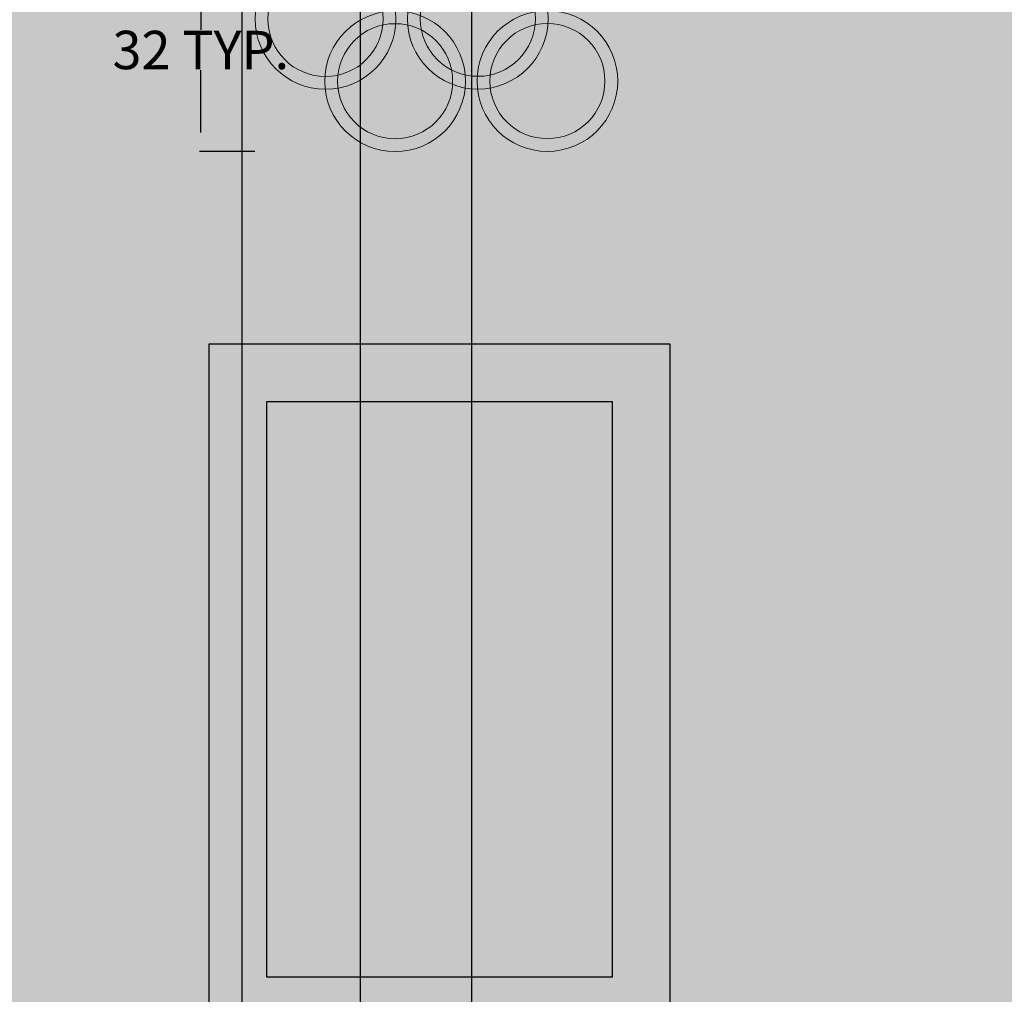
# Model space of a CAD drawing. Units: inches. Extents: x 126 to 726, y 86 to 888.
# Tile 3 of 13: x 270 to 424, y 202 to 354. Entities that reach past the tile are written whole.
import ezdxf

# ---------------------------------------------------------------- set-up
doc = ezdxf.new("R2010")
doc.units = ezdxf.units.IN
doc.header["$MEASUREMENT"] = 0
for name, color, linetype, lineweight in [('A-ANNO-DIMS', 2, 'Continuous', 18), ('A-ELEV-DECO', 7, 'Continuous', 18), ('A-ELEV-PATT', 8, 'Continuous', 13), ('A-GLAZ', 4, 'Continuous', 25)]:
    doc.layers.add(name, color=color, linetype=linetype, lineweight=lineweight)
doc.styles.get("Standard").update_dxf_attribs({"font": 'arial.ttf'})
doc.dimstyles.get("Standard").update_dxf_attribs({"dimtxt": 6, "dimasz": 3, "dimexe": 0.18, "dimexo": 0.0625, "dimgap": 0.09, "dimtad": 0, "dimtih": 1, "dimtoh": 1, "dimdec": 0, "dimzin": 0, "dimdsep": 46, "dimlunit": 3, "dimtxsty": 'Standard', "dimcen": 0.09, "dimadec": 0, "dimazin": 0, "dimtfac": 1, "dimtdec": 0, "dimtofl": 0, "dimtmove": 0, "dimatfit": 3, "dimfxl": 1, "dimtolj": 1, "dimtzin": 0, "dimarcsym": 0})

# ---------------------------------------------------------------- blocks, each defined once
blk = doc.blocks.new('WIN-FRAME')
for points in [[(72, 0), (0, 0), (0, 108), (72, 108)], [(63, 9), (9, 9), (9, 99), (63, 99)]]:
    blk.add_lwpolyline(points, close=True)
blk = doc.blocks.new('MOTIF-RINGS')
for centre, radius in [((11, 20.74), 11), ((34.81, 20.77), 11), ((11, 20.74), 9), ((34.81, 20.77), 9), ((21.88, 11), 11), ((45.69, 11.03), 11), ((45.69, 11.03), 9), ((21.88, 11), 9)]:
    blk.add_circle(centre, radius)
blk = doc.blocks.new('*D9')
at = {"layer": 'A-ANNO-DIMS', "color": 0, "lineweight": -2, "transparency": 16777216}
for p, q in [((306.84, 365.49), (306.84, 374.11)), ((363.53, 365.49), (363.53, 374.11)), ((306.84, 373.93), (303.84, 373.93)), ((360.53, 373.93), (309.84, 373.93))]:
    blk.add_line(p, q, dxfattribs=at)
at = {"layer": 'A-ANNO-DIMS', "color": 0, "transparency": 16777216}
for points in [[(309.84, 374.43), (309.84, 373.43), (306.84, 373.93)], [(360.53, 374.43), (360.53, 373.43), (363.53, 373.93)]]:
    blk.add_solid(points, dxfattribs=at)
at = {"layer": 'Defpoints', "color": 0, "transparency": 16777216}
for p in [(306.84, 373.93), (306.84, 365.42), (363.53, 365.42)]:
    blk.add_point(p, dxfattribs=at)
at = {"layer": 'A-ANNO-DIMS', "color": 0, "transparency": 16777216, "insert": (235.05, 373.93), "char_height": 6, "attachment_point": 5}
blk.add_mtext('\\A1;DECORATIVE RING MOTIF 57 TYP.', dxfattribs=at)
blk = doc.blocks.new('*D10')
at = {"layer": 'A-ANNO-DIMS', "color": 0, "lineweight": -2, "transparency": 16777216}
for p, q in [((306.78, 365.42), (298.16, 365.42)), ((298.34, 362.42), (298.34, 352.7)), ((298.34, 336.66), (298.34, 346.38)), ((306.78, 333.66), (298.16, 333.66))]:
    blk.add_line(p, q, dxfattribs=at)
at = {"layer": 'A-ANNO-DIMS', "color": 0, "transparency": 16777216}
for points in [[(297.84, 362.42), (298.84, 362.42), (298.34, 365.42)], [(297.84, 336.66), (298.84, 336.66), (298.34, 333.66)]]:
    blk.add_solid(points, dxfattribs=at)
at = {"layer": 'Defpoints', "color": 0, "transparency": 16777216}
for p in [(306.84, 365.42), (298.34, 333.66), (306.84, 333.66)]:
    blk.add_point(p, dxfattribs=at)
at = {"layer": 'A-ANNO-DIMS', "color": 0, "transparency": 16777216, "insert": (298.34, 349.54), "char_height": 6, "attachment_point": 5}
blk.add_mtext('\\A1;32 TYP.', dxfattribs=at)
blk = doc.blocks.new('*D13')
at = {"layer": 'A-ANNO-DIMS', "color": 0, "lineweight": -2, "transparency": 16777216}
for p, q in [((665.97, 642.98), (665.97, 90.21)), ((185.97, 126.98), (185.97, 90.21)), ((188.97, 90.39), (419.15, 90.39)), ((662.97, 90.39), (432.8, 90.39))]:
    blk.add_line(p, q, dxfattribs=at)
at = {"layer": 'A-ANNO-DIMS', "color": 0, "transparency": 16777216}
for points in [[(188.97, 90.89), (188.97, 89.89), (185.97, 90.39)], [(662.97, 90.89), (662.97, 89.89), (665.97, 90.39)]]:
    blk.add_solid(points, dxfattribs=at)
at = {"layer": 'Defpoints', "color": 0, "transparency": 16777216}
for p in [(665.97, 643.04), (185.97, 127.04), (665.97, 90.39)]:
    blk.add_point(p, dxfattribs=at)
at = {"layer": 'A-ANNO-DIMS', "color": 0, "transparency": 16777216, "insert": (425.97, 90.39), "char_height": 6, "attachment_point": 5}
blk.add_mtext('\\A1;480', dxfattribs=at)
blk = doc.blocks.new('*D16')
at = {"layer": 'A-ANNO-DIMS', "color": 0, "lineweight": -2, "transparency": 16777216}
for p, q in [((299.6, 425.68), (149.14, 425.68)), ((149.32, 422.68), (149.32, 313.79)), ((149.32, 198.59), (149.32, 307.48)), ((299.6, 195.59), (149.14, 195.59))]:
    blk.add_line(p, q, dxfattribs=at)
at = {"layer": 'A-ANNO-DIMS', "color": 0, "transparency": 16777216}
for points in [[(148.82, 422.68), (149.82, 422.68), (149.32, 425.68)], [(148.82, 198.59), (149.82, 198.59), (149.32, 195.59)]]:
    blk.add_solid(points, dxfattribs=at)
at = {"layer": 'Defpoints', "color": 0, "transparency": 16777216}
for p in [(149.32, 425.68), (299.67, 425.68), (299.67, 195.59)]:
    blk.add_point(p, dxfattribs=at)
at = {"layer": 'A-ANNO-DIMS', "color": 0, "transparency": 16777216, "insert": (149.32, 310.64), "char_height": 6, "attachment_point": 5}
blk.add_mtext('\\A1;230.1', dxfattribs=at)
blk = doc.blocks.new('*D18')
at = {"layer": 'A-ANNO-DIMS', "color": 0, "lineweight": -2, "transparency": 16777216}
for p, q in [((431.28, 395.58), (149.14, 395.58)), ((149.32, 392.58), (149.32, 264.47)), ((149.32, 130.04), (149.32, 258.16)), ((185.91, 127.04), (149.14, 127.04))]:
    blk.add_line(p, q, dxfattribs=at)
at = {"layer": 'A-ANNO-DIMS', "color": 0, "transparency": 16777216}
for points in [[(148.82, 392.58), (149.82, 392.58), (149.32, 395.58)], [(148.82, 130.04), (149.82, 130.04), (149.32, 127.04)]]:
    blk.add_solid(points, dxfattribs=at)
at = {"layer": 'Defpoints', "color": 0, "transparency": 16777216}
for p in [(149.32, 395.58), (431.34, 395.58), (185.97, 127.04)]:
    blk.add_point(p, dxfattribs=at)
at = {"layer": 'A-ANNO-DIMS', "color": 0, "transparency": 16777216, "insert": (149.32, 261.31), "char_height": 6, "attachment_point": 5}
blk.add_mtext('\\A1;268.54', dxfattribs=at)
blk = doc.blocks.new('*D38')
at = {"layer": 'A-ANNO-DIMS', "color": 0, "lineweight": -2, "transparency": 16777216}
for p, q in [((304.8, 168.3), (304.8, 883.87)), ((307.8, 883.69), (320.3, 883.69)), ((323.3, 174.45), (323.3, 883.87)), ((323.3, 883.69), (326.3, 883.69))]:
    blk.add_line(p, q, dxfattribs=at)
at = {"layer": 'A-ANNO-DIMS', "color": 0, "transparency": 16777216}
for points in [[(307.8, 884.19), (307.8, 883.19), (304.8, 883.69)], [(320.3, 884.19), (320.3, 883.19), (323.3, 883.69)]]:
    blk.add_solid(points, dxfattribs=at)
at = {"layer": 'Defpoints', "color": 0, "transparency": 16777216}
for p in [(323.3, 883.69), (323.3, 174.39), (304.8, 168.24)]:
    blk.add_point(p, dxfattribs=at)
at = {"layer": 'A-ANNO-DIMS', "color": 0, "transparency": 16777216, "insert": (338.59, 883.69), "char_height": 6, "attachment_point": 5}
blk.add_mtext('\\A1;18.505', dxfattribs=at)
blk = doc.blocks.new('*D39')
at = {"layer": 'A-ANNO-DIMS', "color": 0, "lineweight": -2, "transparency": 16777216}
for p, q in [((323.3, 174.45), (323.3, 883.87)), ((326.3, 883.69), (337.74, 883.69)), ((340.74, 168.3), (340.74, 883.87)), ((340.74, 883.69), (343.74, 883.69))]:
    blk.add_line(p, q, dxfattribs=at)
at = {"layer": 'A-ANNO-DIMS', "color": 0, "transparency": 16777216}
for points in [[(326.3, 884.19), (326.3, 883.19), (323.3, 883.69)], [(337.74, 884.19), (337.74, 883.19), (340.74, 883.69)]]:
    blk.add_solid(points, dxfattribs=at)
at = {"layer": 'Defpoints', "color": 0, "transparency": 16777216}
for p in [(340.74, 883.69), (323.3, 174.39), (340.74, 168.24)]:
    blk.add_point(p, dxfattribs=at)
at = {"layer": 'A-ANNO-DIMS', "color": 0, "transparency": 16777216, "insert": (355.99, 883.69), "char_height": 6, "attachment_point": 5}
blk.add_mtext('\\A1;17.434', dxfattribs=at)

msp = doc.modelspace()

# ---------------------------------------------------------------- hatches: boundary and pattern name
at = {"layer": 'A-ELEV-PATT'}
h = msp.add_hatch(color=256, dxfattribs=at)
h.dxf.hatch_style = 1
h.paths.add_polyline_path([(437.9749, 499.1312), (485.9749, 499.1312), (485.9749, 501.4423), (437.9749, 501.4423), (437.9749, 513.4423), (485.9749, 513.4423), (485.9749, 515.7534), (437.9749, 515.7534), (437.9749, 527.7534), (485.9749, 527.7534), (485.9749, 530.0646), (437.9749, 530.0646), (437.9749, 542.0646), (485.9749, 542.0646), (485.9749, 544.3757), (437.9749, 544.3757), (437.9749, 556.3757), (485.9749, 556.3757), (485.9749, 558.6868), (437.9749, 558.6868), (437.9749, 570.6868), (485.9749, 570.6868), (485.9749, 572.9979), (437.9749, 572.9979), (437.9749, 584.9979), (485.9749, 584.9979), (485.9749, 587.309), (437.9749, 587.309), (437.9749, 595.0424), (429.9749, 595.0424), (429.9749, 607.0424), (437.9749, 607.0424), (437.9749, 615.9312), (437.9749, 630.2423), (437.9749, 642.2423), (485.9749, 642.2423), (485.9749, 644.5534), (437.9749, 644.5534), (437.9749, 656.5534), (485.9749, 656.5534), (485.9749, 658.8645), (437.9749, 658.8645), (437.9749, 670.8645), (485.9749, 670.8645), (485.9749, 673.1757), (437.9749, 673.1757), (437.9749, 685.1757), (485.9749, 685.1757), (485.9749, 687.4868), (437.9749, 687.4868), (437.9749, 699.4868), (485.9749, 699.4868), (485.9749, 701.7979), (437.9749, 701.7979), (437.9749, 713.7979), (485.9749, 713.7979), (485.9749, 716.109), (437.9749, 716.109), (437.9749, 728.109), (485.9749, 728.109), (485.9749, 730.4201), (437.9749, 730.4201), (437.9749, 742.4201), (485.9749, 742.4201), (485.9749, 744.7312), (437.9749, 744.7312), (437.9749, 756.7312), (485.9749, 756.7312), (485.9749, 759.0423), (437.9749, 759.0423), (437.9749, 771.0423), (485.9749, 771.0423), (485.9749, 773.3534), (437.9749, 773.3534), (437.9749, 785.3534), (485.9749, 785.3534), (485.9749, 787.6645), (437.9749, 787.6645), (437.9749, 799.6645), (485.9749, 799.6645), (485.9749, 801.9756), (437.9749, 801.9756), (437.9749, 811.2868), (485.9749, 811.2868), (485.9749, 813.9756), (437.9749, 813.9756), (437.9749, 825.9756), (485.9749, 825.9756), (485.9749, 835.0424), (233.9749, 835.0424), (233.9749, 606.5846), (185.9749, 606.5846), (185.9749, 597.5846), (233.9749, 597.5846), (233.9749, 585.5846), (185.9749, 585.5846), (185.9749, 580.5846), (233.9749, 580.5846), (233.9749, 568.5846), (185.9749, 568.5846), (185.9749, 563.5846), (431.3386, 563.5846), (431.3386, 545.5846), (233.9749, 545.5846), (233.9749, 413.5846), (431.3386, 413.5846), (431.3386, 395.5846), (185.9749, 395.5846), (185.9749, 386.5846), (233.9749, 386.5846), (233.9749, 374.5846), (185.9749, 374.5846), (185.9749, 369.5846), (233.9749, 369.5846), (233.9749, 357.5846), (185.9749, 357.5846), (185.9749, 352.5846), (233.9749, 352.5846), (233.9749, 340.5846), (185.9749, 340.5846), (185.9749, 331.5846), (233.9749, 331.5846), (233.9749, 127.0424), (485.9749, 127.0424), (485.9749, 129.3535), (437.9749, 129.3535), (437.9749, 141.3535), (485.9749, 141.3535), (485.9749, 143.6646), (437.9749, 143.6646), (437.9749, 155.6646), (485.9749, 155.6646), (485.9749, 157.9757), (437.9749, 157.9757), (437.9749, 169.9757), (485.9749, 169.9757), (485.9749, 172.2868), (437.9749, 172.2868), (437.9749, 184.2868), (485.9749, 184.2868), (485.9749, 186.5979), (437.9749, 186.5979), (437.9749, 198.5979), (485.9749, 198.5979), (485.9749, 200.909), (437.9749, 200.909), (437.9749, 212.909), (485.9749, 212.909), (485.9749, 215.2201), (437.9749, 215.2201), (437.9749, 227.2201), (485.9749, 227.2201), (485.9749, 229.5312), (437.9749, 229.5312), (437.9749, 241.5312), (485.9749, 241.5312), (485.9749, 243.8424), (437.9749, 243.8424), (437.9749, 255.8424), (485.9749, 255.8424), (485.9749, 258.1535), (437.9749, 258.1535), (437.9749, 270.1535), (485.9749, 270.1535), (485.9749, 272.4646), (437.9749, 272.4646), (437.9749, 284.4646), (485.9749, 284.4646), (485.9749, 286.7757), (437.9749, 286.7757), (437.9749, 298.7757), (485.9749, 298.7757), (485.9749, 301.0868), (437.9749, 301.0868), (437.9749, 313.0868), (485.9749, 313.0868), (485.9749, 315.3979), (437.9749, 315.3979), (437.9749, 327.3979), (485.9749, 327.3979), (485.9749, 329.709), (437.9749, 329.709), (437.9749, 341.709), (485.9749, 341.709), (485.9749, 344.0201), (437.9749, 344.0201), (437.9749, 355.0424), (429.9749, 355.0424), (429.9749, 367.0424), (437.9749, 367.0424), (437.9749, 372.6423), (437.9749, 386.9535), (437.9749, 401.2646), (437.9749, 413.2646), (485.9749, 413.2646), (485.9749, 415.5757), (437.9749, 415.5757), (437.9749, 427.5757), (485.9749, 427.5757), (485.9749, 429.8868), (437.9749, 429.8868), (437.9749, 441.8868), (485.9749, 441.8868), (485.9749, 444.1979), (437.9749, 444.1979), (437.9749, 456.1979), (485.9749, 456.1979), (485.9749, 458.509), (437.9749, 458.509), (437.9749, 470.509), (485.9749, 470.509), (485.9749, 472.8201), (437.9749, 472.8201), (437.9749, 484.8201), (485.9749, 484.8201), (485.9749, 487.1312), (437.9749, 487.1312)])
h.paths.add_polyline_path([(299.6658, 533.6845), (371.6658, 533.6845), (371.6658, 425.6845), (299.6658, 425.6845)], flags=16)
h.paths.add_polyline_path([(308.6658, 524.6845), (362.6658, 524.6845), (362.6658, 434.6845), (308.6658, 434.6845)], flags=0)
h.paths.add_polyline_path([(317.7956, 603.3211, -0.4129833), (306.8418, 614.321, -0.94403766), (328.769, 615.5845, -0.04423165), (330.7031, 615.4048, -0.89973713), (352.5798, 615.6161, -0.4129833), (363.5336, 604.6162, -0.94403766), (341.6064, 603.3528, -0.04423165), (339.6723, 603.5324, -0.89973713)], flags=16)
h.paths.add_polyline_path([(319.7228, 604.5846, -0.02633223), (319.7726, 605.5306, -0.47905713), (308.8418, 614.321, -1), (326.8418, 614.321, -0.02633223), (326.7919, 613.375, -0.17413188), (332.826, 612.5948, -0.04918553), (332.6526, 614.3527, -1), (350.6526, 614.3527, -0.02633223), (350.6028, 613.4067, -0.47905713), (361.5336, 604.6162, -1), (343.5336, 604.6162, -0.02633223), (343.5834, 605.5622, -0.17413188), (337.5494, 606.3424, -0.04918553), (337.7228, 604.5846, -1)], flags=0)
h.paths.add_polyline_path([(328.769, 355.6561, -0.04423165), (330.7031, 355.4765, -0.89973713), (352.5798, 355.6878, -0.4129833), (363.5336, 344.6879, -0.94403766), (341.6064, 343.4244, -0.04423165), (339.6723, 343.604, -0.89973713), (317.7956, 343.3927, -0.4129833), (306.8418, 354.3926, -0.94403766)], flags=16)
h.paths.add_polyline_path([(326.8418, 354.3926, -0.02633223), (326.7919, 353.4466, -0.17413188), (332.826, 352.6664, -0.04918553), (332.6526, 354.4243, -1), (350.6526, 354.4243, -0.02633223), (350.6028, 353.4783, -0.47905713), (361.5336, 344.6879, -1), (343.5336, 344.6879, -0.02633223), (343.5834, 345.6339, -0.17413188), (337.5494, 346.4141, -0.04918553), (337.7228, 344.6562, -1), (319.7228, 344.6562, -0.02633223), (319.7726, 345.6022, -0.47905713), (308.8418, 354.3926, -1)], flags=0)
h.paths.add_polyline_path([(299.3189, 655.3527), (299.3189, 763.3527), (371.3189, 763.3527), (371.3189, 655.3527)], flags=16)
h.paths.add_polyline_path([(308.3189, 664.3527), (308.3189, 754.3527), (362.3189, 754.3527), (362.3189, 664.3527)], flags=0)
h.paths.add_polyline_path([(299.6658, 303.5875), (371.6658, 303.5875), (371.6658, 195.5875), (299.6658, 195.5875)], flags=16)
h.paths.add_polyline_path([(308.6658, 294.5875), (362.6658, 294.5875), (362.6658, 204.5875), (308.6658, 204.5875)], flags=0)
h.paths.add_polyline_path([(326.3038, 177.3867), (346.055, 177.3867, -0.41421356), (349.055, 174.3867), (349.055, 171.2378), (363.489, 171.2378, -0.41421356), (366.489, 168.2378), (366.489, 159.7133, -0.41421356), (363.489, 156.7133), (343.7379, 156.7133, -0.41421356), (340.7379, 159.7133), (340.7379, 162.8622), (330.5504, 162.8622), (330.5504, 159.7133, -0.41421356), (327.5504, 156.7133), (307.7992, 156.7133, -0.41421356), (304.7992, 159.7133), (304.7992, 168.2378, -0.41421356), (307.7992, 171.2378), (323.3038, 171.2378), (323.3038, 174.3867, -0.41421356)], flags=16)
h.paths.add_polyline_path([(326.3038, 175.3867), (346.055, 175.3867, -0.41421356), (347.055, 174.3867), (347.055, 169.2378), (363.489, 169.2378, -0.41421356), (364.489, 168.2378), (364.489, 159.7133, -0.41421356), (363.489, 158.7133), (343.7379, 158.7133, -0.41421356), (342.7379, 159.7133), (342.7379, 164.8622), (328.5504, 164.8622), (328.5504, 159.7133, -0.41421356), (327.5504, 158.7133), (307.7992, 158.7133, -0.41421356), (306.7992, 159.7133), (306.7992, 168.2378, -0.41421356), (307.7992, 169.2378), (325.3038, 169.2378), (325.3038, 174.3867, -0.41421356)], flags=0)
h = msp.add_hatch(dxfattribs=at)
h.set_pattern_fill('GRAVEL', color=256, scale=40)
h.paths.add_polyline_path([(437.9749, 642.2423), (485.9749, 642.2423), (485.9749, 644.5534), (437.9749, 644.5534), (437.9749, 656.5534), (485.9749, 656.5534), (485.9749, 658.8645), (437.9749, 658.8645), (437.9749, 670.8645), (485.9749, 670.8645), (485.9749, 673.1757), (437.9749, 673.1757), (437.9749, 685.1757), (485.9749, 685.1757), (485.9749, 687.4868), (437.9749, 687.4868), (437.9749, 699.4868), (485.9749, 699.4868), (485.9749, 701.7979), (437.9749, 701.7979), (437.9749, 713.7979), (485.9749, 713.7979), (485.9749, 716.109), (437.9749, 716.109), (437.9749, 728.109), (485.9749, 728.109), (485.9749, 730.4201), (437.9749, 730.4201), (437.9749, 742.4201), (485.9749, 742.4201), (485.9749, 744.7312), (437.9749, 744.7312), (437.9749, 756.7312), (485.9749, 756.7312), (485.9749, 759.0423), (437.9749, 759.0423), (437.9749, 771.0423), (485.9749, 771.0423), (485.9749, 773.3534), (437.9749, 773.3534), (437.9749, 785.3534), (485.9749, 785.3534), (485.9749, 787.6645), (437.9749, 787.6645), (437.9749, 799.6645), (485.9749, 799.6645), (485.9749, 801.9756), (437.9749, 801.9756), (437.9749, 811.2868), (485.9749, 811.2868), (485.9749, 813.9756), (437.9749, 813.9756), (437.9749, 825.9756), (485.9749, 825.9756), (485.9749, 835.0424), (233.9749, 835.0424), (233.9749, 606.5846), (185.9749, 606.5846), (185.9749, 597.5846), (233.9749, 597.5846), (233.9749, 585.5846), (185.9749, 585.5846), (185.9749, 580.5846), (233.9749, 580.5846), (233.9749, 568.5846), (185.9749, 568.5846), (185.9749, 563.5846), (431.3386, 563.5846), (431.3386, 545.5846), (233.9749, 545.5846), (233.9749, 413.5846), (431.3386, 413.5846), (431.3386, 395.5846), (185.9749, 395.5846), (185.9749, 386.5846), (233.9749, 386.5846), (233.9749, 374.5846), (185.9749, 374.5846), (185.9749, 369.5846), (233.9749, 369.5846), (233.9749, 357.5846), (185.9749, 357.5846), (185.9749, 352.5846), (233.9749, 352.5846), (233.9749, 340.5846), (185.9749, 340.5846), (185.9749, 331.5846), (233.9749, 331.5846), (233.9749, 127.0424), (485.9749, 127.0424), (485.9749, 129.3535), (437.9749, 129.3535), (437.9749, 141.3535), (485.9749, 141.3535), (485.9749, 143.6646), (437.9749, 143.6646), (437.9749, 155.6646), (485.9749, 155.6646), (485.9749, 157.9757), (437.9749, 157.9757), (437.9749, 169.9757), (485.9749, 169.9757), (485.9749, 172.2868), (437.9749, 172.2868), (437.9749, 184.2868), (485.9749, 184.2868), (485.9749, 186.5979), (437.9749, 186.5979), (437.9749, 198.5979), (485.9749, 198.5979), (485.9749, 200.909), (437.9749, 200.909), (437.9749, 212.909), (485.9749, 212.909), (485.9749, 215.2201), (437.9749, 215.2201), (437.9749, 227.2201), (485.9749, 227.2201), (485.9749, 229.5312), (437.9749, 229.5312), (437.9749, 241.5312), (485.9749, 241.5312), (485.9749, 243.8424), (437.9749, 243.8424), (437.9749, 255.8424), (485.9749, 255.8424), (485.9749, 258.1535), (437.9749, 258.1535), (437.9749, 270.1535), (485.9749, 270.1535), (485.9749, 272.4646), (437.9749, 272.4646), (437.9749, 284.4646), (485.9749, 284.4646), (485.9749, 286.7757), (437.9749, 286.7757), (437.9749, 298.7757), (485.9749, 298.7757), (485.9749, 301.0868), (437.9749, 301.0868), (437.9749, 313.0868), (485.9749, 313.0868), (485.9749, 315.3979), (437.9749, 315.3979), (437.9749, 327.3979), (485.9749, 327.3979), (485.9749, 329.709), (437.9749, 329.709), (437.9749, 341.709), (485.9749, 341.709), (485.9749, 344.0201), (437.9749, 344.0201), (437.9749, 355.0424), (429.9749, 355.0424), (429.9749, 367.0424), (437.9749, 367.0424), (437.9749, 372.6423), (437.9749, 386.9535), (437.9749, 401.2646), (437.9749, 413.2646), (485.9749, 413.2646), (485.9749, 415.5757), (437.9749, 415.5757), (437.9749, 427.5757), (485.9749, 427.5757), (485.9749, 429.8868), (437.9749, 429.8868), (437.9749, 441.8868), (485.9749, 441.8868), (485.9749, 444.1979), (437.9749, 444.1979), (437.9749, 456.1979), (485.9749, 456.1979), (485.9749, 458.509), (437.9749, 458.509), (437.9749, 470.509), (485.9749, 470.509), (485.9749, 472.8201), (437.9749, 472.8201), (437.9749, 484.8201), (485.9749, 484.8201), (485.9749, 487.1312), (437.9749, 487.1312), (437.9749, 499.1312), (485.9749, 499.1312), (485.9749, 501.4423), (437.9749, 501.4423), (437.9749, 513.4423), (485.9749, 513.4423), (485.9749, 515.7534), (437.9749, 515.7534), (437.9749, 527.7534), (485.9749, 527.7534), (485.9749, 530.0646), (437.9749, 530.0646), (437.9749, 542.0646), (485.9749, 542.0646), (485.9749, 544.3757), (437.9749, 544.3757), (437.9749, 556.3757), (485.9749, 556.3757), (485.9749, 558.6868), (437.9749, 558.6868), (437.9749, 570.6868), (485.9749, 570.6868), (485.9749, 572.9979), (437.9749, 572.9979), (437.9749, 584.9979), (485.9749, 584.9979), (485.9749, 587.309), (437.9749, 587.309), (437.9749, 595.0424), (429.9749, 595.0424), (429.9749, 607.0424), (437.9749, 607.0424), (437.9749, 615.9312), (437.9749, 630.2423)])
h.paths.add_polyline_path([(371.3189, 655.3527), (299.3189, 655.3527), (299.3189, 763.3527), (371.3189, 763.3527)], flags=16)
h.paths.add_polyline_path([(363.5336, 604.6162, -0.94403766), (341.6064, 603.3528, -0.04423165), (339.6723, 603.5324, -0.89973713), (317.7956, 603.3211, -0.4129833), (306.8418, 614.321, -0.94403766), (328.769, 615.5845, -0.04423165), (330.7031, 615.4048, -0.89973713), (352.5798, 615.6161, -0.4129833)], flags=16)
h.paths.add_polyline_path([(361.5336, 604.6162, -1), (343.5336, 604.6162, -0.02633223), (343.5834, 605.5622, -0.17413188), (337.5494, 606.3424, -0.04918553), (337.7228, 604.5846, -1), (319.7228, 604.5846, -0.02633223), (319.7726, 605.5306, -0.47905713), (308.8418, 614.321, -1), (326.8418, 614.321, -0.02633223), (326.7919, 613.375, -0.17413188), (332.826, 612.5948, -0.04918553), (332.6526, 614.3527, -1), (350.6526, 614.3527, -0.02633223), (350.6028, 613.4067, -0.47905713)], flags=0)
h.paths.add_polyline_path([(362.3189, 664.3527), (308.3189, 664.3527), (308.3189, 754.3527), (362.3189, 754.3527)], flags=0)
h.paths.add_polyline_path([(371.6658, 533.6845), (371.6658, 425.6845), (299.6658, 425.6845), (299.6658, 533.6845)], flags=16)
h.paths.add_polyline_path([(362.6658, 524.6845), (362.6658, 434.6845), (308.6658, 434.6845), (308.6658, 524.6845)], flags=0)
h.paths.add_polyline_path([(352.5798, 355.6878, -0.4129833), (363.5336, 344.6879, -0.94403766), (341.6064, 343.4244, -0.04423165), (339.6723, 343.604, -0.89973713), (317.7956, 343.3927, -0.4129833), (306.8418, 354.3926, -0.94403766), (328.769, 355.6561, -0.04423165), (330.7031, 355.4765, -0.89973713)], flags=16)
h.paths.add_polyline_path([(350.6526, 354.4243, -0.02633223), (350.6028, 353.4783, -0.47905713), (361.5336, 344.6879, -1), (343.5336, 344.6879, -0.02633223), (343.5834, 345.6339, -0.17413188), (337.5494, 346.4141, -0.04918553), (337.7228, 344.6562, -1), (319.7228, 344.6562, -0.02633223), (319.7726, 345.6022, -0.47905713), (308.8418, 354.3926, -1), (326.8418, 354.3926, -0.02633223), (326.7919, 353.4466, -0.17413188), (332.826, 352.6664, -0.04918553), (332.6526, 354.4243, -1)], flags=0)
h.paths.add_polyline_path([(371.6658, 303.5875), (371.6658, 195.5875), (299.6658, 195.5875), (299.6658, 303.5875)], flags=16)
h.paths.add_polyline_path([(362.6658, 294.5875), (362.6658, 204.5875), (308.6658, 204.5875), (308.6658, 294.5875)], flags=0)
h.paths.add_polyline_path([(346.055, 177.3867, -0.41421356), (349.055, 174.3867), (349.055, 171.2378), (363.489, 171.2378, -0.41421356), (366.489, 168.2378), (366.489, 159.7133, -0.41421356), (363.489, 156.7133), (343.7379, 156.7133, -0.41421356), (340.7379, 159.7133), (340.7379, 162.8622), (330.5504, 162.8622), (330.5504, 159.7133, -0.41421356), (327.5504, 156.7133), (307.7992, 156.7133, -0.41421356), (304.7992, 159.7133), (304.7992, 168.2378, -0.41421356), (307.7992, 171.2378), (323.3038, 171.2378), (323.3038, 174.3867, -0.41421356), (326.3038, 177.3867)], flags=16)
h.paths.add_polyline_path([(346.055, 175.3867, -0.41421356), (347.055, 174.3867), (347.055, 169.2378), (363.489, 169.2378, -0.41421356), (364.489, 168.2378), (364.489, 159.7133, -0.41421356), (363.489, 158.7133), (343.7379, 158.7133, -0.41421356), (342.7379, 159.7133), (342.7379, 164.8622), (328.5504, 164.8622), (328.5504, 159.7133, -0.41421356), (327.5504, 158.7133), (307.7992, 158.7133, -0.41421356), (306.7992, 159.7133), (306.7992, 168.2378, -0.41421356), (307.7992, 169.2378), (325.3038, 169.2378), (325.3038, 174.3867, -0.41421356), (326.3038, 175.3867)], flags=0)
h = msp.add_hatch(color=256, dxfattribs=at)
h.dxf.hatch_style = 1
h.paths.add_polyline_path([(343.7379, 171.2378), (347.055, 171.2378), (347.055, 174.3867, 0.41421356), (346.055, 175.3867), (326.3038, 175.3867, 0.41421356), (325.3038, 174.3867), (325.3038, 171.2378), (327.5504, 171.2378, -0.41421356), (330.5504, 168.2378), (330.5504, 164.8622), (340.7379, 164.8622), (340.7379, 168.2378, -0.41421356)])
h.paths.add_polyline_path([(328.5504, 162.8622), (326.3038, 162.8622, -0.41421356), (323.3038, 165.8622), (323.3038, 169.2378), (307.7992, 169.2378, 0.41421356), (306.7992, 168.2378), (306.7992, 159.7133, 0.41421356), (307.7992, 158.7133), (327.5504, 158.7133, 0.41421356), (328.5504, 159.7133)])
h.paths.add_polyline_path([(328.5504, 168.2378, 0.41421356), (327.5504, 169.2378), (325.3038, 169.2378), (325.3038, 165.8622, 0.41421356), (326.3038, 164.8622), (328.5504, 164.8622)], flags=17)
h.paths.add_polyline_path([(364.489, 168.2378, 0.41421356), (363.489, 169.2378), (349.055, 169.2378), (349.055, 165.8622, -0.41421356), (346.055, 162.8622), (342.7379, 162.8622), (342.7379, 159.7133, 0.41421356), (343.7379, 158.7133), (363.489, 158.7133, 0.41421356), (364.489, 159.7133)])
h.paths.add_polyline_path([(347.055, 169.2378), (343.7379, 169.2378, 0.41421356), (342.7379, 168.2378), (342.7379, 164.8622), (346.055, 164.8622, 0.41421356), (347.055, 165.8622)], flags=17)
h.paths.add_polyline_path([(361.5336, 344.6879, 0.4111475), (352.6279, 353.6874, -0.34414474), (343.5998, 343.598, 0.94107412)])
h.paths.add_polyline_path([(332.6665, 354.9249, -0.28599337), (339.6784, 345.6435, 0.05271891), (341.5583, 345.4248, -0.34414474), (350.5864, 355.5141, 0.91517696)])
h.paths.add_polyline_path([(308.8418, 354.3926, 0.4111475), (317.7475, 345.3931, -0.34414474), (326.7756, 355.4825, 0.94107412)])
h.paths.add_polyline_path([(326.7919, 353.4466, 0.32288595), (319.7726, 345.6022, 0.32288595)])
h.paths.add_polyline_path([(330.697, 353.437, 0.05271891), (328.8171, 353.6557, -0.34414474), (319.789, 343.5663, 0.91517696), (337.7088, 344.1556, -0.28599337)])
h.paths.add_polyline_path([(332.826, 352.6664, 0.22909031), (337.5494, 346.4141, 0.22909031)], flags=17)
h.paths.add_polyline_path([(350.6028, 353.4783, 0.32288595), (343.5834, 345.6339, 0.32288595)])
h.paths.add_polyline_path([(332.6665, 614.8533, -0.28599337), (339.6784, 605.5719, 0.05271891), (341.5583, 605.3532, -0.34414474), (350.5864, 615.4425, 0.91517696)])
h.paths.add_polyline_path([(308.8418, 614.321, 0.4111475), (317.7475, 605.3215, -0.34414474), (326.7756, 615.4109, 0.94107412)])
h.paths.add_polyline_path([(337.7088, 604.084, -0.28599337), (330.697, 613.3654, 0.05271891), (328.8171, 613.5841, -0.34414474), (319.789, 603.4947, 0.91517696)])
h.paths.add_polyline_path([(361.5336, 604.6162, 0.4111475), (352.6279, 613.6157, -0.34414474), (343.5998, 603.5264, 0.94107412)])
h.paths.add_polyline_path([(350.6028, 613.4067, 0.32288595), (343.5834, 605.5622, 0.32288595)])
h.paths.add_polyline_path([(332.826, 612.5948, 0.22909031), (337.5494, 606.3424, 0.22909031)], flags=17)
h.paths.add_polyline_path([(326.7919, 613.375, 0.32288595), (319.7726, 605.5306, 0.32288595)])
h = msp.add_hatch(color=256, dxfattribs=at)
h.dxf.hatch_style = 1
h.paths.add_polyline_path([(306.8418, 354.3926, 0.4129833), (317.7956, 343.3927, -0.02878665), (317.7228, 344.6562, -0.0167625), (317.7475, 345.3931, -0.4111475), (308.8418, 354.3926, -0.94107412), (326.7756, 355.4825, -0.04557115), (328.769, 355.6561, 0.94403766)])
h.paths.add_polyline_path([(328.8171, 353.6557, 0.05673494), (326.7919, 353.4466, -0.32288595), (319.7726, 345.6022, 0.02633223), (319.7228, 344.6562, 0.03035736), (319.789, 343.5663, 0.34414474)])
h.paths.add_polyline_path([(326.7919, 353.4466, 0.02633223), (326.8418, 354.3926, 0.03035736), (326.7756, 355.4825, 0.34414474), (317.7475, 345.3931, 0.05673494), (319.7726, 345.6022, -0.32288595)], flags=17)
h.paths.add_polyline_path([(328.769, 355.6561, 0.04557115), (326.7756, 355.4825, -0.03035736), (326.8418, 354.3926, -0.02633223), (326.7919, 353.4466, -0.05673494), (328.8171, 353.6557, 0.0167625), (328.8418, 354.3926, 0.02878665)])
h.paths.add_polyline_path([(330.7031, 355.4765, 0.04423165), (328.769, 355.6561, -0.02878665), (328.8418, 354.3926, -0.0167625), (328.8171, 353.6557, -0.05271891), (330.697, 353.437, -0.022473), (330.6526, 354.4243, -0.02395419)])
h.paths.add_polyline_path([(332.6526, 354.4243, -0.01391386), (332.6665, 354.9249, 0.04645219), (330.7031, 355.4765, 0.02395419), (330.6526, 354.4243, 0.022473), (330.697, 353.437, -0.0631426), (332.826, 352.6664, -0.04918553)])
h.paths.add_polyline_path([(332.826, 352.6664, 0.0631426), (330.697, 353.437, 0.28599337), (337.7088, 344.1556, 0.01391386), (337.7228, 344.6562, 0.04918553), (337.5494, 346.4141, -0.22909031)])
h.paths.add_polyline_path([(332.6665, 354.9249, 0.01391386), (332.6526, 354.4243, 0.04918553), (332.826, 352.6664, -0.22909031), (337.5494, 346.4141, 0.0631426), (339.6784, 345.6435, 0.28599337)])
h.paths.add_polyline_path([(350.5864, 355.5141, -0.04557115), (352.5798, 355.6878, 0.89973713), (330.7031, 355.4765, -0.04645219), (332.6665, 354.9249, -0.91517696)])
h.paths.add_polyline_path([(352.6279, 353.6874, 0.05673494), (350.6028, 353.4783, -0.32288595), (343.5834, 345.6339, 0.02633223), (343.5336, 344.6879, 0.03035736), (343.5998, 343.598, 0.34414474)], flags=17)
h.paths.add_polyline_path([(350.6028, 353.4783, 0.02633223), (350.6526, 354.4243, 0.03035736), (350.5864, 355.5141, 0.34414474), (341.5583, 345.4248, 0.05673494), (343.5834, 345.6339, -0.32288595)])
h.paths.add_polyline_path([(352.5798, 355.6878, 0.04557115), (350.5864, 355.5141, -0.03035736), (350.6526, 354.4243, -0.02633223), (350.6028, 353.4783, -0.05673494), (352.6279, 353.6874, 0.0167625), (352.6526, 354.4243, 0.02878665)])
h.paths.add_polyline_path([(343.5834, 345.6339, -0.05673494), (341.5583, 345.4248, 0.0167625), (341.5336, 344.6879, 0.02878665), (341.6064, 343.4244, 0.04557115), (343.5998, 343.598, -0.03035736), (343.5336, 344.6879, -0.02633223)])
h.paths.add_polyline_path([(339.6784, 345.6435, -0.0631426), (337.5494, 346.4141, -0.04918553), (337.7228, 344.6562, -0.01391386), (337.7088, 344.1556, 0.04645219), (339.6723, 343.604, 0.02395419), (339.7228, 344.6562, 0.022473)])
h.paths.add_polyline_path([(341.5336, 344.6879, -0.0167625), (341.5583, 345.4248, -0.05271891), (339.6784, 345.6435, -0.022473), (339.7228, 344.6562, -0.02395419), (339.6723, 343.604, 0.04423165), (341.6064, 343.4244, -0.02878665)])
h.paths.add_polyline_path([(339.6723, 343.604, -0.04645219), (337.7088, 344.1556, -0.91517696), (319.789, 343.5663, -0.04557115), (317.7956, 343.3927, 0.89973713)])
h.paths.add_polyline_path([(343.5998, 343.598, -0.04557115), (341.6064, 343.4244, 0.94403766), (363.5336, 344.6879, 0.4129833), (352.5798, 355.6878, -0.02878665), (352.6526, 354.4243, -0.0167625), (352.6279, 353.6874, -0.4111475), (361.5336, 344.6879, -0.94107412)])
h.paths.add_polyline_path([(319.7228, 344.6562, -0.02633223), (319.7726, 345.6022, -0.05673494), (317.7475, 345.3931, 0.0167625), (317.7228, 344.6562, 0.02878665), (317.7956, 343.3927, 0.04557115), (319.789, 343.5663, -0.03035736)])
h = msp.add_hatch(color=256, dxfattribs=at)
h.dxf.hatch_style = 1
h.paths.add_polyline_path([(371.6658, 303.5875), (299.6658, 303.5875), (299.6658, 195.5875), (371.6658, 195.5875)])
h.paths.add_polyline_path([(362.6658, 294.5875), (362.6658, 204.5875), (308.6658, 204.5875), (308.6658, 294.5875)], flags=16)
h.paths.add_polyline_path([(366.489, 159.7133), (366.489, 168.2378, 0.41421356), (363.489, 171.2378), (349.055, 171.2378), (349.055, 169.2378), (363.489, 169.2378, -0.41421356), (364.489, 168.2378), (364.489, 159.7133, -0.41421356), (363.489, 158.7133), (343.7379, 158.7133, -0.41421356), (342.7379, 159.7133), (342.7379, 162.8622), (340.7379, 162.8622), (340.7379, 159.7133, 0.41421356), (343.7379, 156.7133), (363.489, 156.7133, 0.41421356)])
h.paths.add_polyline_path([(349.055, 171.2378), (347.055, 171.2378), (347.055, 169.2378), (349.055, 169.2378)], flags=17)
h.paths.add_polyline_path([(349.055, 169.2378), (347.055, 169.2378), (347.055, 165.8622, -0.41421356), (346.055, 164.8622), (342.7379, 164.8622), (342.7379, 162.8622), (346.055, 162.8622, 0.41421356), (349.055, 165.8622)], flags=17)
h.paths.add_polyline_path([(342.7379, 164.8622), (340.7379, 164.8622), (340.7379, 162.8622), (342.7379, 162.8622)], flags=17)
h.paths.add_polyline_path([(342.7379, 168.2378, -0.41421356), (343.7379, 169.2378), (347.055, 169.2378), (347.055, 171.2378), (343.7379, 171.2378, 0.41421356), (340.7379, 168.2378), (340.7379, 164.8622), (342.7379, 164.8622)], flags=17)
h.paths.add_polyline_path([(349.055, 174.3867, 0.41421356), (346.055, 177.3867), (326.3038, 177.3867, 0.41421356), (323.3038, 174.3867), (323.3038, 171.2378), (325.3038, 171.2378), (325.3038, 174.3867, -0.41421356), (326.3038, 175.3867), (346.055, 175.3867, -0.41421356), (347.055, 174.3867), (347.055, 171.2378), (349.055, 171.2378)])
h.paths.add_polyline_path([(327.5504, 171.2378), (325.3038, 171.2378), (325.3038, 169.2378), (327.5504, 169.2378, -0.41421356), (328.5504, 168.2378), (328.5504, 164.8622), (330.5504, 164.8622), (330.5504, 168.2378, 0.41421356)], flags=17)
h.paths.add_polyline_path([(325.3038, 171.2378), (323.3038, 171.2378), (323.3038, 169.2378), (325.3038, 169.2378)], flags=17)
h.paths.add_polyline_path([(325.3038, 169.2378), (323.3038, 169.2378), (323.3038, 165.8622, 0.41421356), (326.3038, 162.8622), (328.5504, 162.8622), (328.5504, 164.8622), (326.3038, 164.8622, -0.41421356), (325.3038, 165.8622)], flags=17)
h.paths.add_polyline_path([(330.5504, 164.8622), (328.5504, 164.8622), (328.5504, 162.8622), (330.5504, 162.8622)], flags=17)
h.paths.add_polyline_path([(340.7379, 164.8622), (330.5504, 164.8622), (330.5504, 162.8622), (340.7379, 162.8622)])
h.paths.add_polyline_path([(330.5504, 162.8622), (328.5504, 162.8622), (328.5504, 159.7133, -0.41421356), (327.5504, 158.7133), (307.7992, 158.7133, -0.41421356), (306.7992, 159.7133), (306.7992, 168.2378, -0.41421356), (307.7992, 169.2378), (323.3038, 169.2378), (323.3038, 171.2378), (307.7992, 171.2378, 0.41421356), (304.7992, 168.2378), (304.7992, 159.7133, 0.41421356), (307.7992, 156.7133), (327.5504, 156.7133, 0.41421356), (330.5504, 159.7133)])
at = {"layer": 'A-GLAZ'}
h = msp.add_hatch(color=256, dxfattribs=at)
h.dxf.hatch_style = 1
h.paths.add_polyline_path([(362.6658, 294.5875), (308.6658, 294.5875), (308.6658, 204.5875), (362.6658, 204.5875)])

# ---------------------------------------------------------------- block references
at = {"layer": 'A-ELEV-DECO', "rotation": 180}
msp.add_blockref('MOTIF-RINGS', (363.5334, 365.4239), dxfattribs=at)
at = {"layer": 'A-GLAZ'}
msp.add_blockref('WIN-FRAME', (299.6659, 195.5878), dxfattribs=at)

# ---------------------------------------------------------------- dimensions: what is measured, and where the dimension line sits
at = {"layer": 'A-ANNO-DIMS'}
for base, p1, p2, override, picture, middle in [((323.3038, 883.6924), (304.7992, 168.2378), (323.3038, 174.3867), {"dimdec": 3, "dimlfac": 1, "dimrnd": 0, "dimzin": 0, "dimdsep": 46, "dimlunit": 2}, '*D38', (338.5882, 883.6924)), ((340.7379, 883.6924), (323.3038, 174.3867), (340.7379, 168.2378), {"dimdec": 3, "dimlfac": 1, "dimrnd": 0, "dimzin": 0, "dimdsep": 46, "dimlunit": 2}, '*D39', (355.9875, 883.6924)), ((665.9749, 90.3924), (185.9749, 127.0424), (665.9749, 643.0424), {"dimdec": 0, "dimlfac": 1, "dimrnd": 0, "dimzin": 0, "dimdsep": 46, "dimlunit": 2}, '*D13', (425.9749, 90.3924))]:
    dim = msp.add_linear_dim(base=base, p1=p1, p2=p2, dimstyle='Standard', override=override, dxfattribs=at)
    dim.commit()
    dim.dimension.update_dxf_attribs({"geometry": picture, "text_midpoint": middle})
for base, p1, p2, override, picture, middle in [((149.3249, 425.6845), (299.6658, 195.5875), (299.6658, 425.6845), {"dimdec": 1, "dimlfac": 1, "dimrnd": 0, "dimzin": 0, "dimdsep": 46, "dimlunit": 2}, '*D16', (149.3249, 310.636)), ((149.3249, 395.5846), (185.9749, 127.0424), (431.3386, 395.5846), {"dimdec": 2, "dimlfac": 1, "dimrnd": 0, "dimzin": 0, "dimdsep": 46, "dimlunit": 2}, '*D18', (149.3249, 261.3135))]:
    dim = msp.add_linear_dim(base=base, p1=p1, p2=p2, angle=90, dimstyle='Standard', override=override, dxfattribs=at)
    dim.commit()
    dim.dimension.update_dxf_attribs({"geometry": picture, "text_midpoint": middle})
for base, p1, p2, angle, text, picture, middle in [((306.8418, 373.9281), (363.5336, 365.4243), (306.8418, 365.4243), 180, 'DECORATIVE RING MOTIF <> TYP.', '*D9', (235.0465, 373.9281)), ((298.338, 333.6562), (306.8418, 365.4243), (306.8418, 333.6562), 270, '<> TYP.', '*D10', (298.338, 349.5402))]:
    dim = msp.add_linear_dim(base=base, p1=p1, p2=p2, angle=angle, text=text, dimstyle='Standard', override={"dimdec": 0, "dimlfac": 1, "dimrnd": 0, "dimzin": 0, "dimdsep": 46, "dimlunit": 2}, dxfattribs=at)
    dim.commit()
    dim.dimension.update_dxf_attribs({"geometry": picture, "text_midpoint": middle})

doc.saveas('drawing.dxf')
